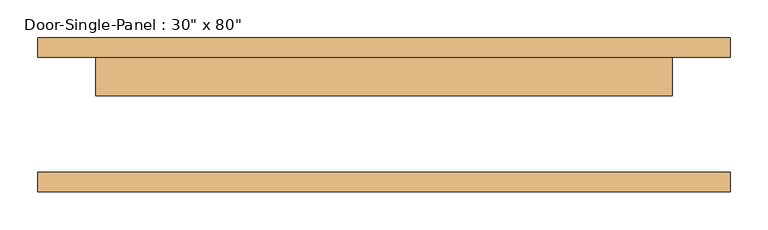
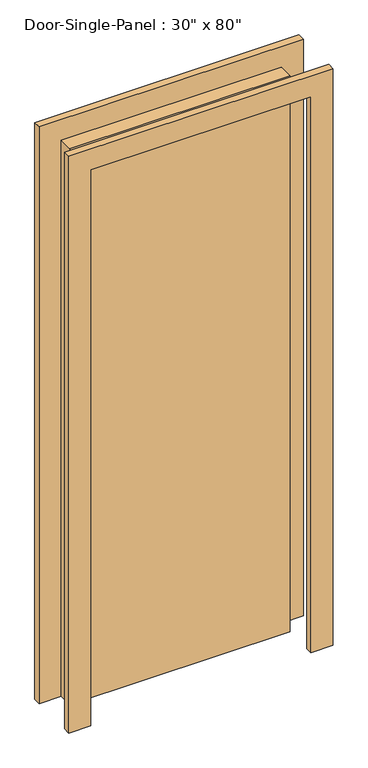
"""IFC4 building model written with IfcOpenShell, lengths in millimetres: door geometry."""

from ifc_helpers import new_model, si_unit, frame, origin, origin_with_axes, place, context, project, spatial, polyline, outline, extrude, source, transform, mapped, element, save


def door_c31ea698(model_context):
    return source(origin(), model_context, "Body", "SweptSolid", [
        extrude(outline(polyline([(381.0, 25.4), (-381.0, 25.4), (-381.0, 76.2), (381.0, 76.2), (381.0, 25.4)])), origin_with_axes(), (0.0, 0.0, 1.0), 2032.0),
        extrude(outline(polyline([(2108.2, -457.2), (0.0, -457.2), (0.0, -381.0), (2032.0, -381.0), (2032.0, 381.0), (0.0, 381.0), (0.0, 457.2), (2108.2, 457.2), (2108.2, -457.2)])), frame((0.0, 76.2, 0.0), z_axis=(0.0, 1.0, 0.0), x_axis=(0.0, 0.0, 1.0)), (0.0, 0.0, 1.0), 25.4),
        extrude(outline(polyline([(2108.2, 457.2), (2108.2, -457.2), (0.0, -457.2), (0.0, -381.0), (2032.0, -381.0), (2032.0, 381.0), (0.0, 381.0), (0.0, 457.2), (2108.2, 457.2)])), frame((0.0, -101.6, 0.0), z_axis=(0.0, 1.0, 0.0), x_axis=(0.0, 0.0, 1.0)), (0.0, 0.0, 1.0), 25.4),
    ])


if __name__ == "__main__":
    model = new_model("IFC4")
    model_context = context("Model", 3, world=origin())
    ifc_project = project(units=[si_unit("LENGTHUNIT", "METRE", prefix="MILLI")], contexts=[model_context])
    site = spatial("IfcSite", under=ifc_project)
    building = spatial("IfcBuilding", under=site)
    placement = place(None, origin())
    door_shape = door_c31ea698(model_context)
    element("IfcDoor", 1, ObjectType="Door-Single-Panel : 30\" x 80\"", at=placement, inside=building, context=model_context, shape_type="MappedRepresentation", body=[
        mapped(door_shape, transform((0.0, 0.0, 0.0), x_axis=(1.0, 0.0, 0.0), y_axis=(0.0, 1.0, 0.0), z_axis=(0.0, 0.0, 1.0))),
    ])
    save(model, "model.ifc")

# Revit data of these elements
# Type "Door-Single-Panel : 30\" x 80\""
#   Type Mark = "11"
#   Construction Type Id = "DOOR"
#   Assembly Code = "C1020300"
#   Analytic Construction = "Wooden"
#   Thickness = 0' - 2"
#   Thermal Resistance (R) = 2.5876 (h·ft²·°F)/BTU
#   Swing Angle [instance default] = 90.00°
#   Heat Transfer Coefficient (U) = 0.3865 BTU/(h·ft²·°F)
#   Height = 6' - 8"
#   Trim Projection Ext = 0' - 1"
#   Trim Projection Int = 0' - 1"
#   Trim Width = 0' - 3"
#   Width = 2' - 6"
#   Define Thermal Properties by = 1
#   Panel Material = Wood - Birch - Solid Stained Light Low Gloss
#   Trim Material = Paint - Sienna
#   Visual Light Transmittance = 0
#   Solar Heat Gain Coefficient = 0
#   Function = (empty or 0)
#   Wall Closure = (empty or 0)
# Element 1 (IfcDoor, "Door-Single-Panel : 30\" x 80\"")
#   Materials on its faces: "Paint - Sienna", "Wood - Birch - Solid Stained Light Low Gloss"
# Materials
#   "Wood - Birch - Solid Stained Light Low Gloss": class "Wood", colour RGB 210 159 95, transparency 0, Cost = 0
#   "Paint - Sienna": colour RGB 118 70 51, transparency 0, Cost = 0
